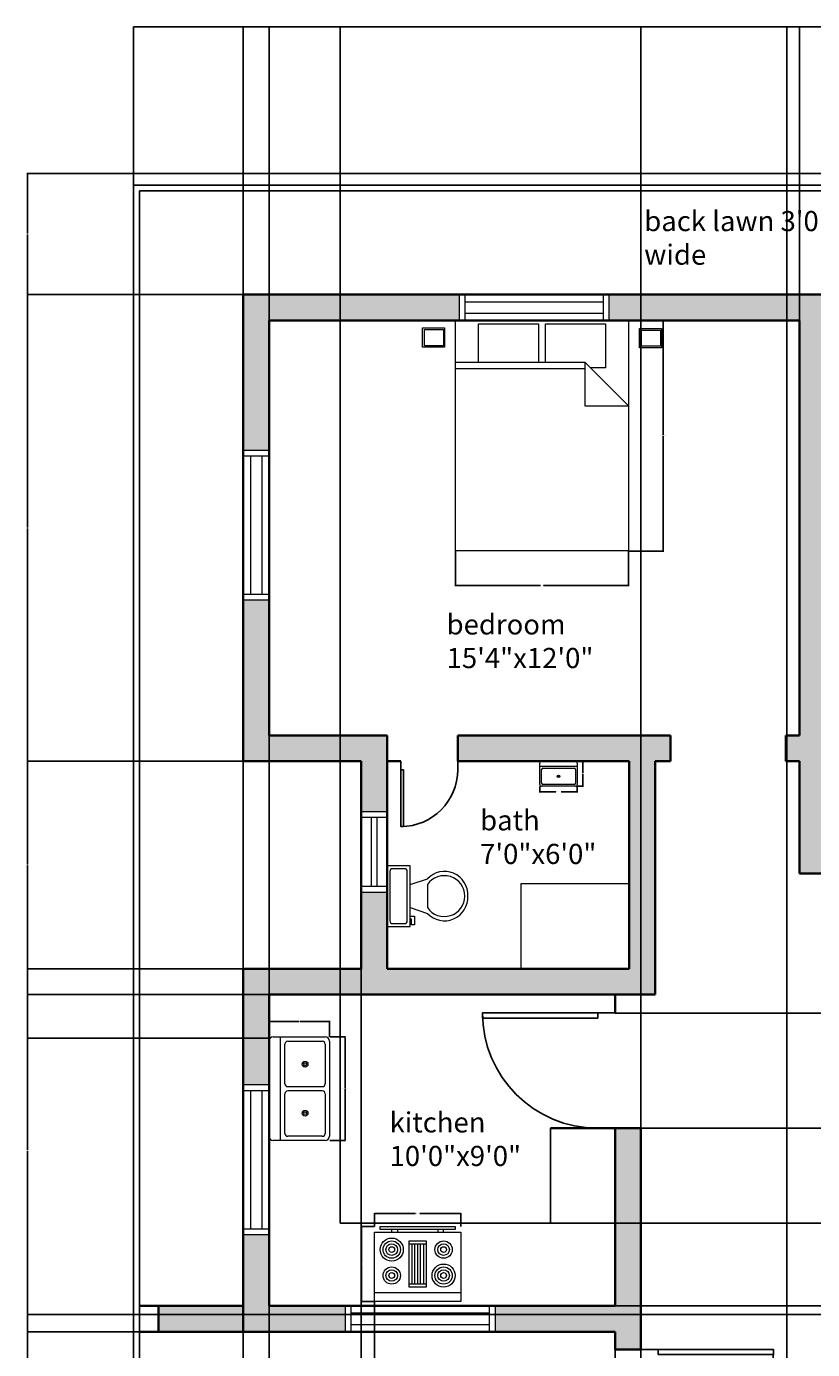
# Model space of a CAD drawing. Units: inches. Extents: x 1801 to 2333, y 478 to 1258.
# Tile 2 of 3: x 1801 to 2074, y 798 to 1258. Entities that reach past the tile are written whole.
import ezdxf

# ---------------------------------------------------------------- set-up
doc = ezdxf.new("R2010")
doc.units = ezdxf.units.IN
doc.header["$MEASUREMENT"] = 0
for name, color, linetype, lineweight in [('A-ANNO-DIMS', 2, 'Continuous', 18), ('A-AREA-IDEN', 7, 'Continuous', 18), ('A-DOOR', 4, 'Continuous', 25), ('A-EQPM', 8, 'Continuous', 18), ('A-FLOR-CASE', 8, 'Continuous', 25), ('A-FLOR-FIXT', 9, 'Continuous', 18), ('A-FURN', 8, 'Continuous', 18), ('A-GLAZ', 4, 'Continuous', 18), ('A-WALL', 7, 'Continuous', 35), ('A-WALL-PATT', 252, 'Continuous', 13), ('C-PROP', 3, 'Continuous', 25)]:
    doc.layers.add(name, color=color, linetype=linetype, lineweight=lineweight)
doc.styles.get("Standard").update_dxf_attribs({"font": 'arial.ttf'})
doc.dimstyles.get("Standard").update_dxf_attribs({"dimtxt": 0.18, "dimasz": 0.18, "dimexe": 0.18, "dimexo": 0.0625, "dimgap": 0.09, "dimtad": 0, "dimtih": 1, "dimtoh": 1, "dimdec": 0, "dimzin": 0, "dimdsep": 46, "dimlunit": 3, "dimtxsty": 'Standard', "dimcen": 0.09, "dimadec": 0, "dimazin": 0, "dimtfac": 1, "dimtdec": 0, "dimtofl": 0, "dimtmove": 0, "dimatfit": 3, "dimfxl": 1, "dimtolj": 1, "dimtzin": 0, "dimarcsym": 0})

# ---------------------------------------------------------------- blocks, each defined once
blk = doc.blocks.new('*U2')
for p, q in [((0, 0), (0, -6)), ((40, 0), (40, -6))]:
    blk.add_line(p, q)
blk.add_lwpolyline([(0, 0), (0, 40), (1.75, 40), (1.75, 0)], close=True)
blk.add_arc((0, 0), 40, 0, 90)
blk = doc.blocks.new('*U6')
for p, q in [((241.3, -152.4), (241.3, -50.8)), ((-254, -215.9), (-203.2, -215.9)), ((-254, -241.3), (-254, -215.9)), ((-203.2, -215.9), (-203.2, -203.2)), ((-177.8, -203.2), (-177.8, -241.3)), ((-101.6, -203.2), (-152.4, -355.6)), ((101.6, -203.2), (152.4, -355.6)), ((-177.8, -241.3), (-254, -241.3)), ((101.6, -355.6), (-101.6, -355.6))]:
    blk.add_line(p, q)
blk.add_lwpolyline([(266.7, -203.2), (266.7, 0), (-266.7, 0), (-266.7, -203.2)], close=True)
for points in [[(-241.3, -50.8), (-241.3, -152.4)], [(215.9, -25.4), (-215.9, -25.4)], [(-215.9, -177.8), (215.9, -177.8)]]:
    blk.add_lwpolyline(points)
for centre, radius, start, end in [((-219.075, -47.625), 22.45064, 81.8699, 188.1301), ((219.075, -47.625), 22.45064, 351.8699, 98.1301), ((-219.075, -155.575), 22.45064, 171.869898, 278.1301), ((219.075, -155.575), 22.45064, 261.8699, 8.1301), ((-12.12088, -505.93752), 205.61935, 133.01722, 273.38), ((0.94996, -504.77674), 181.02486, 124.50543, 269.7), ((-0.94742, -504.77674), 181.02486, 270.3, 55.4946), ((12.12342, -505.93752), 205.61935, 266.62, 46.9828)]:
    blk.add_arc(centre, radius, start, end)
blk = doc.blocks.new('Bed - Queen')
for p, q in [((0, -80.00003), (0, 0)), ((0, 0), (59.99999, 0)), ((59.99999, 0), (59.99999, -80.00003)), ((7.99999, -1.2), (28.79998, -1.2)), ((7.99999, -14.4), (7.99999, -1.2)), ((28.79998, -1.2), (28.79998, -14.4)), ((31.19999, -1.2), (51.99999, -1.2)), ((31.19999, -14.4), (31.19999, -1.2)), ((51.99999, -1.2), (51.99999, -16.4)), ((0, -14.4), (44.8, -14.4)), ((44.8, -16.8), (0, -16.8)), ((59.99999, -29.6), (44.8, -14.4)), ((44.8, -14.4), (44.8, -29.6)), ((51.99999, -16.4), (46.79936, -16.4)), ((44.8, -29.6), (59.99999, -29.6)), ((59.99999, -80.00003), (0, -80.00003))]:
    blk.add_line(p, q)
blk = doc.blocks.new('Sink-double - 36 in top')
for p, q in [((-18, -4), (18, -4)), ((-0.75, -18.5), (-0.75, -6.5)), ((0.75, -6.5), (0.75, -18.5))]:
    blk.add_line(p, q)
for points in [[(-16.5, 0), (16.5, 0)], [(-18, -19.5), (-18, -1.5)], [(18, -1.5), (18, -19.5)], [(-16.5, -18.5), (-16.5, -6.5)], [(-15.5, -5.5), (-1.75, -5.5)], [(1.75, -5.5), (15.5, -5.5)], [(16.5, -6.5), (16.5, -18.5)], [(16.5, -21), (-16.5, -21)], [(-1.75, -19.5), (-15.5, -19.5)], [(15.5, -19.5), (1.75, -19.5)]]:
    blk.add_lwpolyline(points)
for centre, radius in [((-8.5, -12.5), 1), ((-8.5, -12.5), 0.5), ((8.5, -12.5), 1), ((8.5, -12.5), 0.5)]:
    blk.add_circle(centre, radius)
for centre, radius, start, end in [((-16.5, -1.5), 1.5, 90, 180), ((16.5, -1.5), 1.5, 0, 90), ((-15.5, -6.5), 1, 90, 180), ((-1.75, -6.5), 1, 0, 90), ((1.75, -6.5), 1, 90, 180), ((15.5, -6.5), 1, 0, 90), ((-16.5, -19.5), 1.5, 180, 270), ((-15.5, -18.5), 1, 180, 270), ((-1.75, -18.5), 1, 270, 0), ((1.75, -18.5), 1, 180, 270), ((15.5, -18.5), 1, 270, 0), ((16.5, -19.5), 1.5, 270, 0)]:
    blk.add_arc(centre, radius, start, end)
blk = doc.blocks.new('Range-Oven - 30 in top')
for p, q in [((0, -3), (30, -3)), ((12, -6), (18, -6)), ((13, -20), (13, -6)), ((14, -6), (14, -20)), ((15, -20), (15, -6)), ((16, -6), (16, -20)), ((17, -20), (17, -6)), ((18, -20), (12, -20)), ((6, -24), (6, -25)), ((8, -25), (8, -24)), ((22, -25), (22, -24)), ((24, -24), (24, -25))]:
    blk.add_line(p, q)
for points in [[(0, -24), (0, 0), (30, 0), (30, -24)], [(12, -21), (12, -5), (18, -5), (18, -21)], [(2, -26), (2, -25), (28, -25), (28, -26)]]:
    blk.add_lwpolyline(points, close=True)
for centre, radius in [((6, -9), 4), ((6, -9), 3), ((6, -9), 2), ((6, -9), 1), ((24, -9), 3), ((24, -9), 2), ((24, -9), 1), ((6, -18), 3), ((6, -18), 2), ((6, -18), 1), ((24, -18), 4), ((24, -18), 3), ((24, -18), 2), ((24, -18), 1)]:
    blk.add_circle(centre, radius)
blk = doc.blocks.new('Sink-single - 30 in top')
blk.add_line((-15, -3.999996), (15, -3.999996))
for points in [[(-13.5, 0), (13.5, 0)], [(-15, -18.499996), (-15, -1.5)], [(-13.5, -17.499996), (-13.5, -6.499996)], [(-12.5, -5.499996), (12.5, -5.499996)], [(13.5, -6.499996), (13.5, -17.499996)], [(15, -1.5), (15, -18.499996)], [(13.5, -19.999996), (-13.5, -19.999996)], [(12.5, -18.499996), (-12.5, -18.499996)]]:
    blk.add_lwpolyline(points)
for radius in [1, 0.5]:
    blk.add_circle((0, -11.999996), radius)
for centre, radius, start, end in [((-13.5, -1.5), 1.5, 90, 180), ((-12.5, -6.499996), 1, 90, 180), ((12.5, -6.499996), 1, 0, 90), ((13.5, -1.5), 1.5, 0, 90), ((-13.5, -18.499996), 1.5, 180, 270), ((-12.5, -17.499996), 1, 180, 270), ((12.5, -17.499996), 1, 270, 0), ((13.5, -18.499996), 1.5, 270, 0)]:
    blk.add_arc(centre, radius, start, end)
blk = doc.blocks.new('WIN-48IN')
for p, q in [((0, 0), (0, 9)), ((2, 0), (2, 9)), ((2, 6.5), (50, 6.5)), ((50, 0), (50, 9)), ((52, 0), (52, 9)), ((2, 2.5), (50, 2.5))]:
    blk.add_line(p, q)
blk = doc.blocks.new('WIN-24IN')
for p, q in [((9, 28), (0, 28)), ((9, 26), (0, 26)), ((3.5, 26), (3.5, 2)), ((5.5, 26), (5.5, 2)), ((9, 2), (0, 2)), ((9, 0), (0, 0))]:
    blk.add_line(p, q)
blk = doc.blocks.new('BEDSIDE-STAND')
for points in [[(0, 6.71), (7.61, 6.71), (7.61, 0), (0, 0)], [(0.62, 6.12), (7.2, 6.12), (7.2, 0.48), (0.62, 0.48)]]:
    blk.add_lwpolyline(points, close=True)
blk = doc.blocks.new('*D23')
at = {"layer": 'A-ANNO-DIMS', "color": 0, "lineweight": -2, "transparency": 16777216}
for p, q in [((2010.04, 1155.47), (2022.16, 1155.47)), ((2021.98, 1155.29), (2021.98, 1115.66)), ((2021.98, 1075.65), (2021.98, 1115.29)), ((2010.04, 1075.47), (2022.16, 1075.47))]:
    blk.add_line(p, q, dxfattribs=at)
at = {"layer": 'A-ANNO-DIMS', "color": 0, "transparency": 16777216}
for points in [[(2021.95, 1155.29), (2022.01, 1155.29), (2021.98, 1155.47)], [(2021.95, 1075.65), (2022.01, 1075.65), (2021.98, 1075.47)]]:
    blk.add_solid(points, dxfattribs=at)
at = {"layer": 'Defpoints', "color": 0, "transparency": 16777216}
for p in [(2009.98, 1155.47), (2021.98, 1155.47), (2009.98, 1075.47)]:
    blk.add_point(p, dxfattribs=at)
at = {"layer": 'A-ANNO-DIMS', "color": 0, "transparency": 16777216, "insert": (2021.98, 1115.47), "char_height": 0.18, "attachment_point": 5}
blk.add_mtext('\\A1;QUEEN BED 80 TYP.', dxfattribs=at)
blk = doc.blocks.new('*D24')
at = {"layer": 'A-ANNO-DIMS', "color": 0, "lineweight": -2, "transparency": 16777216}
for p, q in [((1949.98, 1075.41), (1949.98, 1063.29)), ((2009.98, 1075.41), (2009.98, 1063.29)), ((1950.16, 1063.47), (1979.45, 1063.47)), ((2009.8, 1063.47), (1980.51, 1063.47))]:
    blk.add_line(p, q, dxfattribs=at)
at = {"layer": 'A-ANNO-DIMS', "color": 0, "transparency": 16777216}
for points in [[(1950.16, 1063.5), (1950.16, 1063.44), (1949.98, 1063.47)], [(2009.8, 1063.5), (2009.8, 1063.44), (2009.98, 1063.47)]]:
    blk.add_solid(points, dxfattribs=at)
at = {"layer": 'Defpoints', "color": 0, "transparency": 16777216}
for p in [(1949.98, 1075.47), (2009.98, 1075.47), (2009.98, 1063.47)]:
    blk.add_point(p, dxfattribs=at)
at = {"layer": 'A-ANNO-DIMS', "color": 0, "transparency": 16777216, "insert": (1979.98, 1063.47), "char_height": 0.18, "attachment_point": 5}
blk.add_mtext('\\A1;60 TYP.', dxfattribs=at)
blk = doc.blocks.new('*D29')
at = {"layer": 'A-ANNO-DIMS', "color": 0, "lineweight": -2, "transparency": 16777216}
for p, q in [((1979.19, 993.75), (1979.19, 991.68)), ((1992.19, 993.75), (1992.19, 991.68)), ((1979.37, 991.86), (1984.75, 991.86)), ((1992.01, 991.86), (1986.62, 991.86))]:
    blk.add_line(p, q, dxfattribs=at)
at = {"layer": 'A-ANNO-DIMS', "color": 0, "transparency": 16777216}
for points in [[(1979.37, 991.89), (1979.37, 991.83), (1979.19, 991.86)], [(1992.01, 991.89), (1992.01, 991.83), (1992.19, 991.86)]]:
    blk.add_solid(points, dxfattribs=at)
at = {"layer": 'Defpoints', "color": 0, "transparency": 16777216}
for p in [(1979.19, 993.81), (1992.19, 993.81), (1992.19, 991.86)]:
    blk.add_point(p, dxfattribs=at)
at = {"layer": 'A-ANNO-DIMS', "color": 0, "transparency": 16777216, "insert": (1985.69, 991.86), "char_height": 0.18, "attachment_point": 5}
blk.add_mtext('\\A1;BASIN 13 TYP.', dxfattribs=at)
blk = doc.blocks.new('*D30')
at = {"layer": 'A-ANNO-DIMS', "color": 0, "lineweight": -2, "transparency": 16777216}
for p, q in [((1992.25, 1002.47), (1994.32, 1002.47)), ((1994.14, 1002.29), (1994.14, 998.32)), ((1994.14, 993.99), (1994.14, 997.96)), ((1992.25, 993.81), (1994.32, 993.81))]:
    blk.add_line(p, q, dxfattribs=at)
at = {"layer": 'A-ANNO-DIMS', "color": 0, "transparency": 16777216}
for points in [[(1994.11, 1002.29), (1994.17, 1002.29), (1994.14, 1002.47)], [(1994.11, 993.99), (1994.17, 993.99), (1994.14, 993.81)]]:
    blk.add_solid(points, dxfattribs=at)
at = {"layer": 'Defpoints', "color": 0, "transparency": 16777216}
for p in [(1992.19, 1002.47), (1994.14, 1002.47), (1992.19, 993.81)]:
    blk.add_point(p, dxfattribs=at)
at = {"layer": 'A-ANNO-DIMS', "color": 0, "transparency": 16777216, "insert": (1994.14, 998.14), "char_height": 0.18, "attachment_point": 5}
blk.add_mtext('\\A1;9 TYP.', dxfattribs=at)
blk = doc.blocks.new('*D31')
at = {"layer": 'A-ANNO-DIMS', "color": 0, "lineweight": -2, "transparency": 16777216}
for p, q in [((1921.82, 841.04), (1921.82, 845.65)), ((1922, 845.47), (1936.13, 845.47)), ((1951.64, 845.47), (1937.52, 845.47)), ((1951.82, 841.04), (1951.82, 845.65))]:
    blk.add_line(p, q, dxfattribs=at)
at = {"layer": 'A-ANNO-DIMS', "color": 0, "transparency": 16777216}
for points in [[(1922, 845.5), (1922, 845.44), (1921.82, 845.47)], [(1951.64, 845.5), (1951.64, 845.44), (1951.82, 845.47)]]:
    blk.add_solid(points, dxfattribs=at)
at = {"layer": 'Defpoints', "color": 0, "transparency": 16777216}
for p in [(1921.82, 845.47), (1921.82, 840.97), (1951.82, 840.97)]:
    blk.add_point(p, dxfattribs=at)
at = {"layer": 'A-ANNO-DIMS', "color": 0, "transparency": 16777216, "insert": (1936.82, 845.47), "char_height": 0.18, "attachment_point": 5}
blk.add_mtext('\\A1;RANGE 30', dxfattribs=at)
blk = doc.blocks.new('*D32')
at = {"layer": 'A-ANNO-DIMS', "color": 0, "lineweight": -2, "transparency": 16777216}
for p, q in [((1921.76, 840.97), (1917.14, 840.97)), ((1917.32, 840.79), (1917.32, 828.16)), ((1917.32, 815.15), (1917.32, 827.79)), ((1921.76, 814.97), (1917.14, 814.97))]:
    blk.add_line(p, q, dxfattribs=at)
at = {"layer": 'A-ANNO-DIMS', "color": 0, "transparency": 16777216}
for points in [[(1917.29, 840.79), (1917.35, 840.79), (1917.32, 840.97)], [(1917.29, 815.15), (1917.35, 815.15), (1917.32, 814.97)]]:
    blk.add_solid(points, dxfattribs=at)
at = {"layer": 'Defpoints', "color": 0, "transparency": 16777216}
for p in [(1921.82, 840.97), (1917.32, 814.97), (1921.82, 814.97)]:
    blk.add_point(p, dxfattribs=at)
at = {"layer": 'A-ANNO-DIMS', "color": 0, "transparency": 16777216, "insert": (1917.32, 827.97), "char_height": 0.18, "attachment_point": 5}
blk.add_mtext('\\A1;26', dxfattribs=at)
blk = doc.blocks.new('*D33')
at = {"layer": 'A-ANNO-DIMS', "color": 0, "lineweight": -2, "transparency": 16777216}
for p, q in [((1906.31, 906.81), (1911.83, 906.81)), ((1911.65, 906.63), (1911.65, 889)), ((1911.65, 870.99), (1911.65, 888.63)), ((1906.31, 870.81), (1911.83, 870.81))]:
    blk.add_line(p, q, dxfattribs=at)
at = {"layer": 'A-ANNO-DIMS', "color": 0, "transparency": 16777216}
for points in [[(1911.62, 906.63), (1911.68, 906.63), (1911.65, 906.81)], [(1911.62, 870.99), (1911.68, 870.99), (1911.65, 870.81)]]:
    blk.add_solid(points, dxfattribs=at)
at = {"layer": 'Defpoints', "color": 0, "transparency": 16777216}
for p in [(1906.25, 906.81), (1911.65, 906.81), (1906.25, 870.81)]:
    blk.add_point(p, dxfattribs=at)
at = {"layer": 'A-ANNO-DIMS', "color": 0, "transparency": 16777216, "insert": (1911.65, 888.81), "char_height": 0.18, "attachment_point": 5}
blk.add_mtext('\\A1;DOUBLE SINK 36', dxfattribs=at)
blk = doc.blocks.new('*D34')
at = {"layer": 'A-ANNO-DIMS', "color": 0, "lineweight": -2, "transparency": 16777216}
for p, q in [((1885.25, 906.88), (1885.25, 912.39)), ((1885.43, 912.21), (1895.55, 912.21)), ((1906.07, 912.21), (1895.95, 912.21)), ((1906.25, 906.88), (1906.25, 912.39))]:
    blk.add_line(p, q, dxfattribs=at)
at = {"layer": 'A-ANNO-DIMS', "color": 0, "transparency": 16777216}
for points in [[(1885.43, 912.24), (1885.43, 912.18), (1885.25, 912.21)], [(1906.07, 912.24), (1906.07, 912.18), (1906.25, 912.21)]]:
    blk.add_solid(points, dxfattribs=at)
at = {"layer": 'Defpoints', "color": 0, "transparency": 16777216}
for p in [(1885.25, 912.21), (1885.25, 906.81), (1906.25, 906.81)]:
    blk.add_point(p, dxfattribs=at)
at = {"layer": 'A-ANNO-DIMS', "color": 0, "transparency": 16777216, "insert": (1895.75, 912.21), "char_height": 0.18, "attachment_point": 5}
blk.add_mtext('\\A1;21', dxfattribs=at)
blk = doc.blocks.new('*D35')
at = {"layer": 'A-ANNO-DIMS', "color": 0, "lineweight": -2, "transparency": 16777216}
for p, q in [((1838.29, 1202.54), (1838.29, 1257.55)), ((1838.47, 1257.37), (2067, 1257.37)), ((2296.11, 1257.37), (2067.58, 1257.37)), ((2296.29, 1206.54), (2296.29, 1257.55))]:
    blk.add_line(p, q, dxfattribs=at)
at = {"layer": 'A-ANNO-DIMS', "color": 0, "transparency": 16777216}
for points in [[(1838.47, 1257.4), (1838.47, 1257.34), (1838.29, 1257.37)], [(2296.11, 1257.4), (2296.11, 1257.34), (2296.29, 1257.37)]]:
    blk.add_solid(points, dxfattribs=at)
at = {"layer": 'Defpoints', "color": 0, "transparency": 16777216}
for p in [(2296.29, 1257.37), (2296.29, 1206.47), (1838.29, 1202.47)]:
    blk.add_point(p, dxfattribs=at)
at = {"layer": 'A-ANNO-DIMS', "color": 0, "transparency": 16777216, "insert": (2067.29, 1257.37), "char_height": 0.18, "attachment_point": 5}
blk.add_mtext('\\A1;458', dxfattribs=at)
blk = doc.blocks.new('*D37')
at = {"layer": 'A-ANNO-DIMS', "color": 0, "lineweight": -2, "transparency": 16777216}
for p, q in [((1840.29, 804.41), (1840.29, 478.11)), ((2005.29, 804.41), (2005.29, 478.11)), ((1840.47, 478.29), (1922.51, 478.29)), ((2005.11, 478.29), (1923.07, 478.29))]:
    blk.add_line(p, q, dxfattribs=at)
at = {"layer": 'A-ANNO-DIMS', "color": 0, "transparency": 16777216}
for points in [[(1840.47, 478.32), (1840.47, 478.26), (1840.29, 478.29)], [(2005.11, 478.32), (2005.11, 478.26), (2005.29, 478.29)]]:
    blk.add_solid(points, dxfattribs=at)
at = {"layer": 'Defpoints', "color": 0, "transparency": 16777216}
for p in [(1840.29, 804.47), (2005.29, 804.47), (2005.29, 478.29)]:
    blk.add_point(p, dxfattribs=at)
at = {"layer": 'A-ANNO-DIMS', "color": 0, "transparency": 16777216, "insert": (1922.79, 478.29), "char_height": 0.18, "attachment_point": 5}
blk.add_mtext('\\A1;165', dxfattribs=at)
blk = doc.blocks.new('*D39')
at = {"layer": 'A-ANNO-DIMS', "color": 0, "lineweight": -2, "transparency": 16777216}
for p, q in [((1876.29, 1164.54), (1876.29, 1257.55)), ((1876.47, 1257.37), (1972.51, 1257.37)), ((2069.11, 1257.37), (1973.07, 1257.37)), ((2069.29, 1155.54), (2069.29, 1257.55))]:
    blk.add_line(p, q, dxfattribs=at)
at = {"layer": 'A-ANNO-DIMS', "color": 0, "transparency": 16777216}
for points in [[(1876.47, 1257.4), (1876.47, 1257.34), (1876.29, 1257.37)], [(2069.11, 1257.4), (2069.11, 1257.34), (2069.29, 1257.37)]]:
    blk.add_solid(points, dxfattribs=at)
at = {"layer": 'Defpoints', "color": 0, "transparency": 16777216}
for p in [(2069.29, 1257.37), (1876.29, 1164.47), (2069.29, 1155.47)]:
    blk.add_point(p, dxfattribs=at)
at = {"layer": 'A-ANNO-DIMS', "color": 0, "transparency": 16777216, "insert": (1972.79, 1257.37), "char_height": 0.18, "attachment_point": 5}
blk.add_mtext('\\A1;193', dxfattribs=at)
blk = doc.blocks.new('*D40')
at = {"layer": 'A-ANNO-DIMS', "color": 0, "lineweight": -2, "transparency": 16777216}
for p, q in [((2069.29, 1155.54), (2069.29, 1257.55)), ((2069.47, 1257.37), (2131.51, 1257.37)), ((2194.11, 1257.37), (2132.07, 1257.37)), ((2194.29, 1164.54), (2194.29, 1257.55))]:
    blk.add_line(p, q, dxfattribs=at)
at = {"layer": 'A-ANNO-DIMS', "color": 0, "transparency": 16777216}
for points in [[(2069.47, 1257.4), (2069.47, 1257.34), (2069.29, 1257.37)], [(2194.11, 1257.4), (2194.11, 1257.34), (2194.29, 1257.37)]]:
    blk.add_solid(points, dxfattribs=at)
at = {"layer": 'Defpoints', "color": 0, "transparency": 16777216}
for p in [(2194.29, 1257.37), (2194.29, 1164.47), (2069.29, 1155.47)]:
    blk.add_point(p, dxfattribs=at)
at = {"layer": 'A-ANNO-DIMS', "color": 0, "transparency": 16777216, "insert": (2131.79, 1257.37), "char_height": 0.18, "attachment_point": 5}
blk.add_mtext('\\A1;125', dxfattribs=at)
blk = doc.blocks.new('*D42')
at = {"layer": 'A-ANNO-DIMS', "color": 0, "lineweight": -2, "transparency": 16777216}
for p, q in [((1876.23, 1002.47), (1801.26, 1002.47)), ((1801.44, 1002.29), (1801.44, 966.66)), ((1801.44, 930.65), (1801.44, 966.29)), ((1876.23, 930.47), (1801.26, 930.47))]:
    blk.add_line(p, q, dxfattribs=at)
at = {"layer": 'A-ANNO-DIMS', "color": 0, "transparency": 16777216}
for points in [[(1801.41, 1002.29), (1801.47, 1002.29), (1801.44, 1002.47)], [(1801.41, 930.65), (1801.47, 930.65), (1801.44, 930.47)]]:
    blk.add_solid(points, dxfattribs=at)
at = {"layer": 'Defpoints', "color": 0, "transparency": 16777216}
for p in [(1801.44, 1002.47), (1876.29, 1002.47), (1876.29, 930.47)]:
    blk.add_point(p, dxfattribs=at)
at = {"layer": 'A-ANNO-DIMS', "color": 0, "transparency": 16777216, "insert": (1801.44, 966.47), "char_height": 0.18, "attachment_point": 5}
blk.add_mtext('\\A1;72', dxfattribs=at)
blk = doc.blocks.new('*D43')
at = {"layer": 'A-ANNO-DIMS', "color": 0, "lineweight": -2, "transparency": 16777216}
for p, q in [((1876.23, 1164.47), (1801.26, 1164.47)), ((1801.44, 1164.29), (1801.44, 1083.66)), ((1801.44, 1002.65), (1801.44, 1083.29)), ((1876.23, 1002.47), (1801.26, 1002.47))]:
    blk.add_line(p, q, dxfattribs=at)
at = {"layer": 'A-ANNO-DIMS', "color": 0, "transparency": 16777216}
for points in [[(1801.41, 1164.29), (1801.47, 1164.29), (1801.44, 1164.47)], [(1801.41, 1002.65), (1801.47, 1002.65), (1801.44, 1002.47)]]:
    blk.add_solid(points, dxfattribs=at)
at = {"layer": 'Defpoints', "color": 0, "transparency": 16777216}
for p in [(1801.44, 1164.47), (1876.29, 1164.47), (1876.29, 1002.47)]:
    blk.add_point(p, dxfattribs=at)
at = {"layer": 'A-ANNO-DIMS', "color": 0, "transparency": 16777216, "insert": (1801.44, 1083.47), "char_height": 0.18, "attachment_point": 5}
blk.add_mtext('\\A1;162', dxfattribs=at)
blk = doc.blocks.new('*D44')
at = {"layer": 'A-ANNO-DIMS', "color": 0, "lineweight": -2, "transparency": 16777216}
for p, q in [((2194.23, 1206.47), (1801.26, 1206.47)), ((1801.44, 1206.29), (1801.44, 1185.66)), ((1801.44, 1164.65), (1801.44, 1185.29)), ((2194.23, 1164.47), (1801.26, 1164.47))]:
    blk.add_line(p, q, dxfattribs=at)
at = {"layer": 'A-ANNO-DIMS', "color": 0, "transparency": 16777216}
for points in [[(1801.41, 1206.29), (1801.47, 1206.29), (1801.44, 1206.47)], [(1801.41, 1164.65), (1801.47, 1164.65), (1801.44, 1164.47)]]:
    blk.add_solid(points, dxfattribs=at)
at = {"layer": 'Defpoints', "color": 0, "transparency": 16777216}
for p in [(1801.44, 1206.47), (2194.29, 1206.47), (2194.29, 1164.47)]:
    blk.add_point(p, dxfattribs=at)
at = {"layer": 'A-ANNO-DIMS', "color": 0, "transparency": 16777216, "insert": (1801.44, 1185.47), "char_height": 0.18, "attachment_point": 5}
blk.add_mtext('\\A1;42', dxfattribs=at)
blk = doc.blocks.new('*D45')
at = {"layer": 'A-ANNO-DIMS', "color": 0, "lineweight": -2, "transparency": 16777216}
for p, q in [((1876.29, 1002.41), (1876.29, 478.11)), ((1917.2, 1002.41), (1917.2, 478.11)), ((1876.47, 478.29), (1896.36, 478.29)), ((1917.02, 478.29), (1897.12, 478.29))]:
    blk.add_line(p, q, dxfattribs=at)
at = {"layer": 'A-ANNO-DIMS', "color": 0, "transparency": 16777216}
for points in [[(1876.47, 478.32), (1876.47, 478.26), (1876.29, 478.29)], [(1917.02, 478.32), (1917.02, 478.26), (1917.2, 478.29)]]:
    blk.add_solid(points, dxfattribs=at)
at = {"layer": 'Defpoints', "color": 0, "transparency": 16777216}
for p in [(1876.29, 1002.47), (1917.2, 1002.47), (1917.2, 478.29)]:
    blk.add_point(p, dxfattribs=at)
at = {"layer": 'A-ANNO-DIMS', "color": 0, "transparency": 16777216, "insert": (1896.74, 478.29), "char_height": 0.18, "attachment_point": 5}
blk.add_mtext('\\A1;40.91', dxfattribs=at)
blk = doc.blocks.new('*D48')
at = {"layer": 'A-ANNO-DIMS', "color": 0, "lineweight": -2, "transparency": 16777216}
for p, q in [((2147.23, 810.47), (1801.26, 810.47)), ((1801.44, 810.29), (1801.44, 789.42)), ((1801.44, 768.17), (1801.44, 789.05)), ((2147.23, 767.99), (1801.26, 767.99))]:
    blk.add_line(p, q, dxfattribs=at)
at = {"layer": 'A-ANNO-DIMS', "color": 0, "transparency": 16777216}
for points in [[(1801.41, 810.29), (1801.47, 810.29), (1801.44, 810.47)], [(1801.41, 768.17), (1801.47, 768.17), (1801.44, 767.99)]]:
    blk.add_solid(points, dxfattribs=at)
at = {"layer": 'Defpoints', "color": 0, "transparency": 16777216}
for p in [(1801.44, 810.47), (2147.29, 810.47), (2147.29, 767.99)]:
    blk.add_point(p, dxfattribs=at)
at = {"layer": 'A-ANNO-DIMS', "color": 0, "transparency": 16777216, "insert": (1801.44, 789.23), "char_height": 0.18, "attachment_point": 5}
blk.add_mtext('\\A1;42.48', dxfattribs=at)
blk = doc.blocks.new('*D49')
at = {"layer": 'A-ANNO-DIMS', "color": 0, "lineweight": -2, "transparency": 16777216}
for p, q in [((1876.23, 930.47), (1801.26, 930.47)), ((1801.44, 930.29), (1801.44, 867.66)), ((1801.44, 804.65), (1801.44, 867.29)), ((1876.23, 804.47), (1801.26, 804.47))]:
    blk.add_line(p, q, dxfattribs=at)
at = {"layer": 'A-ANNO-DIMS', "color": 0, "transparency": 16777216}
for points in [[(1801.41, 930.29), (1801.47, 930.29), (1801.44, 930.47)], [(1801.41, 804.65), (1801.47, 804.65), (1801.44, 804.47)]]:
    blk.add_solid(points, dxfattribs=at)
at = {"layer": 'Defpoints', "color": 0, "transparency": 16777216}
for p in [(1801.44, 930.47), (1876.29, 930.47), (1876.29, 804.47)]:
    blk.add_point(p, dxfattribs=at)
at = {"layer": 'A-ANNO-DIMS', "color": 0, "transparency": 16777216, "insert": (1801.44, 867.47), "char_height": 0.18, "attachment_point": 5}
blk.add_mtext('\\A1;126', dxfattribs=at)
blk = doc.blocks.new('*D50')
at = {"layer": 'A-ANNO-DIMS', "color": 0, "lineweight": -2, "transparency": 16777216}
for p, q in [((1885.29, 921.54), (1885.29, 1257.55)), ((1885.47, 1257.37), (1897.18, 1257.37)), ((1909.81, 1257.37), (1898.1, 1257.37)), ((1909.99, 921.54), (1909.99, 1257.55))]:
    blk.add_line(p, q, dxfattribs=at)
at = {"layer": 'A-ANNO-DIMS', "color": 0, "transparency": 16777216}
for points in [[(1885.47, 1257.4), (1885.47, 1257.34), (1885.29, 1257.37)], [(1909.81, 1257.4), (1909.81, 1257.34), (1909.99, 1257.37)]]:
    blk.add_solid(points, dxfattribs=at)
at = {"layer": 'Defpoints', "color": 0, "transparency": 16777216}
for p in [(1909.99, 1257.37), (1885.29, 921.47), (1909.99, 921.47)]:
    blk.add_point(p, dxfattribs=at)
at = {"layer": 'A-ANNO-DIMS', "color": 0, "transparency": 16777216, "insert": (1897.64, 1257.37), "char_height": 0.18, "attachment_point": 5}
blk.add_mtext('\\A1;24.704', dxfattribs=at)
blk = doc.blocks.new('*D51')
at = {"layer": 'A-ANNO-DIMS', "color": 0, "lineweight": -2, "transparency": 16777216}
for p, q in [((1982.97, 842.2), (2333.32, 842.2)), ((2333.14, 842.02), (2333.14, 828.02)), ((2333.14, 813.65), (2333.14, 827.65)), ((2005.35, 813.47), (2333.32, 813.47))]:
    blk.add_line(p, q, dxfattribs=at)
at = {"layer": 'A-ANNO-DIMS', "color": 0, "transparency": 16777216}
for points in [[(2333.11, 842.02), (2333.17, 842.02), (2333.14, 842.2)], [(2333.11, 813.65), (2333.17, 813.65), (2333.14, 813.47)]]:
    blk.add_solid(points, dxfattribs=at)
at = {"layer": 'Defpoints', "color": 0, "transparency": 16777216}
for p in [(1982.91, 842.2), (2005.29, 813.47), (2333.14, 813.47)]:
    blk.add_point(p, dxfattribs=at)
at = {"layer": 'A-ANNO-DIMS', "color": 0, "transparency": 16777216, "insert": (2333.14, 827.84), "char_height": 0.18, "attachment_point": 5}
blk.add_mtext('\\A1;28.72', dxfattribs=at)
blk = doc.blocks.new('*D52')
at = {"layer": 'A-ANNO-DIMS', "color": 0, "lineweight": -2, "transparency": 16777216}
for p, q in [((1885.29, 813.41), (1885.29, 478.11)), ((1921.82, 814.91), (1921.82, 478.11)), ((1885.47, 478.29), (1903.09, 478.29)), ((1921.64, 478.29), (1904.02, 478.29))]:
    blk.add_line(p, q, dxfattribs=at)
at = {"layer": 'A-ANNO-DIMS', "color": 0, "transparency": 16777216}
for points in [[(1885.47, 478.32), (1885.47, 478.26), (1885.29, 478.29)], [(1921.64, 478.32), (1921.64, 478.26), (1921.82, 478.29)]]:
    blk.add_solid(points, dxfattribs=at)
at = {"layer": 'Defpoints', "color": 0, "transparency": 16777216}
for p in [(1885.29, 813.47), (1921.82, 814.97), (1921.82, 478.29)]:
    blk.add_point(p, dxfattribs=at)
at = {"layer": 'A-ANNO-DIMS', "color": 0, "transparency": 16777216, "insert": (1903.56, 478.29), "char_height": 0.18, "attachment_point": 5}
blk.add_mtext('\\A1;36.534', dxfattribs=at)
blk = doc.blocks.new('*D53')
at = {"layer": 'A-ANNO-DIMS', "color": 0, "lineweight": -2, "transparency": 16777216}
for p, q in [((1885.23, 921.47), (1801.26, 921.47)), ((1801.44, 921.29), (1801.44, 914.11)), ((1801.44, 906.55), (1801.44, 913.74)), ((1885.63, 906.37), (1801.26, 906.37))]:
    blk.add_line(p, q, dxfattribs=at)
at = {"layer": 'A-ANNO-DIMS', "color": 0, "transparency": 16777216}
for points in [[(1801.41, 921.29), (1801.47, 921.29), (1801.44, 921.47)], [(1801.41, 906.55), (1801.47, 906.55), (1801.44, 906.37)]]:
    blk.add_solid(points, dxfattribs=at)
at = {"layer": 'Defpoints', "color": 0, "transparency": 16777216}
for p in [(1885.29, 921.47), (1801.44, 906.37), (1885.69, 906.37)]:
    blk.add_point(p, dxfattribs=at)
at = {"layer": 'A-ANNO-DIMS', "color": 0, "transparency": 16777216, "insert": (1801.44, 913.92), "char_height": 0.18, "attachment_point": 5}
blk.add_mtext('\\A1;15.1', dxfattribs=at)
blk = doc.blocks.new('*D54')
at = {"layer": 'A-ANNO-DIMS', "color": 0, "lineweight": -2, "transparency": 16777216}
for p, q in [((2005.35, 915.1), (2333.32, 915.1)), ((2333.14, 914.92), (2333.14, 895.29)), ((2333.14, 875.28), (2333.14, 894.92)), ((2005.35, 875.1), (2333.32, 875.1))]:
    blk.add_line(p, q, dxfattribs=at)
at = {"layer": 'A-ANNO-DIMS', "color": 0, "transparency": 16777216}
for points in [[(2333.11, 914.92), (2333.17, 914.92), (2333.14, 915.1)], [(2333.11, 875.28), (2333.17, 875.28), (2333.14, 875.1)]]:
    blk.add_solid(points, dxfattribs=at)
at = {"layer": 'Defpoints', "color": 0, "transparency": 16777216}
for p in [(2005.29, 915.1), (2333.14, 915.1), (2005.29, 875.1)]:
    blk.add_point(p, dxfattribs=at)
at = {"layer": 'A-ANNO-DIMS', "color": 0, "transparency": 16777216, "insert": (2333.14, 895.1), "char_height": 0.18, "attachment_point": 5}
blk.add_mtext('\\A1;40', dxfattribs=at)
blk = doc.blocks.new('*D55')
at = {"layer": 'A-ANNO-DIMS', "color": 0, "lineweight": -2, "transparency": 16777216}
for p, q in [((2014.29, 702.54), (2014.29, 1257.55)), ((2014.47, 1257.37), (2039.21, 1257.37)), ((2064.75, 1257.37), (2040, 1257.37)), ((2064.93, 702.54), (2064.93, 1257.55))]:
    blk.add_line(p, q, dxfattribs=at)
at = {"layer": 'A-ANNO-DIMS', "color": 0, "transparency": 16777216}
for points in [[(2014.47, 1257.4), (2014.47, 1257.34), (2014.29, 1257.37)], [(2064.75, 1257.4), (2064.75, 1257.34), (2064.93, 1257.37)]]:
    blk.add_solid(points, dxfattribs=at)
at = {"layer": 'Defpoints', "color": 0, "transparency": 16777216}
for p in [(2064.93, 1257.37), (2014.29, 702.47), (2064.93, 702.47)]:
    blk.add_point(p, dxfattribs=at)
at = {"layer": 'A-ANNO-DIMS', "color": 0, "transparency": 16777216, "insert": (2039.61, 1257.37), "char_height": 0.18, "attachment_point": 5}
blk.add_mtext('\\A1;50.64', dxfattribs=at)

msp = doc.modelspace()

# ---------------------------------------------------------------- hatches: boundary and pattern name
at = {"layer": 'A-WALL-PATT'}
h = msp.add_hatch(color=256, dxfattribs=at)
h.dxf.hatch_style = 1
h.paths.add_polyline_path([(1951.2881, 1164.4747), (1876.2881, 1164.4747), (1876.2881, 1110.5123), (1885.2881, 1110.5123), (1885.2881, 1155.4747), (1951.2881, 1155.4747)])
h.paths.add_polyline_path([(2126.8707, 1164.4747), (2003.2881, 1164.4747), (2003.2881, 1155.4747), (2069.2881, 1155.4747), (2069.2881, 1011.4747), (2064.4791, 1011.4747), (2064.4791, 1002.4747), (2069.2881, 1002.4747), (2069.2881, 963.4747), (2078.3234, 963.4747), (2086.6392, 963.4747), (2086.6392, 972.4747), (2078.3234, 972.4747), (2078.2881, 1002.4747), (2078.2881, 1155.4747), (2126.8707, 1155.4747)])
h.paths.add_polyline_path([(2194.2881, 1164.4747), (2178.8707, 1164.4747), (2178.8707, 1155.4747), (2194.2881, 1155.4747)])
h.paths.add_polyline_path([(2203.2881, 1206.4747), (2194.2881, 1206.4747), (2194.2881, 1156.4812), (2203.2881, 1156.4812)])
h.paths.add_polyline_path([(2296.2881, 1206.4747), (2287.2881, 1206.4747), (2287.2881, 1187.4062), (2296.2881, 1187.4062)])
h = msp.add_hatch(color=256, dxfattribs=at)
h.dxf.hatch_style = 1
h.paths.add_polyline_path([(1926.1982, 1011.4747), (1885.2881, 1011.4747), (1885.2881, 1058.5123), (1876.2881, 1058.5123), (1876.2881, 1002.4747), (1917.1982, 1002.4747), (1917.1982, 984.9747), (1926.1982, 984.9747)])
h.paths.add_polyline_path([(2024.4791, 1011.4747), (1950.7011, 1011.4747), (1950.7011, 1002.4747), (2010.1982, 1002.4747), (2010.1982, 930.4747), (1972.6781, 930.4747), (1926.1982, 930.4747), (1926.1982, 956.9747), (1917.1982, 956.9747), (1917.1982, 930.4747), (1876.2881, 930.4747), (1876.2881, 890.2272), (1885.2881, 890.2272), (1885.2881, 921.4747), (2014.2881, 921.4747), (2019.1982, 921.4747), (2019.1982, 1002.4747), (2024.4791, 1002.4747)])
h.paths.add_polyline_path([(1911.7913, 813.4747), (1885.2881, 813.4747), (1885.2881, 838.2272), (1876.2881, 838.2272), (1876.2881, 804.4747), (1911.7913, 804.4747)])
h.paths.add_polyline_path([(1876.2881, 813.4747), (1846.9543, 813.4747), (1846.9543, 804.4747), (1876.2881, 804.4747)])
h.paths.add_polyline_path([(2014.2881, 875.105), (2005.2881, 875.105), (2005.2881, 813.4747), (1963.7913, 813.4747), (1963.7913, 804.4747), (2005.2881, 804.4747), (2005.2881, 798.2841), (2014.2881, 798.2841), (2014.2881, 804.4747)])

# ---------------------------------------------------------------- linework, layer by layer
at = {"layer": 'A-FLOR-CASE'}
for p, q in [((1909.9916, 921.4747), (1909.9916, 842.1967)), ((1982.9092, 842.1967), (1982.9092, 875.105)), ((1909.9916, 842.1967), (1982.9092, 842.1967))]:
    msp.add_line(p, q, dxfattribs=at)
at = {"layer": 'A-FLOR-FIXT'}
msp.add_lwpolyline([(2010.1982, 930.4747), (1972.6781, 930.4747), (1972.6781, 960.0868), (2010.1982, 960.0868)], close=True, dxfattribs=at)
at = {"layer": 'A-WALL'}
for p, q in [((1876.2881, 1164.4747), (2194.2881, 1164.4747)), ((1876.2881, 1002.4747), (1876.2881, 1164.4747)), ((1885.2881, 1155.4747), (2069.2881, 1155.4747)), ((1885.2881, 1011.4747), (1885.2881, 1155.4747)), ((2069.2881, 1011.4747), (2069.2881, 1155.4747)), ((1885.2881, 1011.4747), (1926.1982, 1011.4747)), ((1926.1982, 1011.4747), (1926.1982, 930.4747)), ((1950.7011, 1011.4747), (2024.4791, 1011.4747)), ((1950.7011, 1002.4747), (1950.7011, 1011.4747)), ((2024.4791, 1011.4747), (2024.4791, 1002.4747)), ((2064.4791, 1011.4747), (2064.4791, 1002.4747)), ((2064.4791, 1011.4747), (2069.2881, 1011.4747)), ((1876.2881, 1002.4747), (1917.1982, 1002.4747)), ((1917.1982, 1002.4747), (1917.1982, 930.4747)), ((1926.1982, 1002.4747), (1931.0142, 1002.4747)), ((1950.7011, 1002.4747), (2010.1982, 1002.4747)), ((2010.1982, 1002.4747), (2010.1982, 930.4747)), ((2019.1982, 1002.4747), (2019.1982, 921.4747)), ((2019.1982, 1002.4747), (2024.4791, 1002.4747)), ((2064.4791, 1002.4747), (2069.2881, 1002.4747)), ((2069.2881, 1002.4747), (2069.2881, 963.4747)), ((2069.2881, 963.4747), (2078.3234, 963.4747)), ((1876.2881, 930.4747), (1917.1982, 930.4747)), ((1876.2881, 804.4747), (1876.2881, 930.4747)), ((1926.1982, 930.4747), (2010.1982, 930.4747)), ((1885.2881, 921.4747), (2014.2881, 921.4747)), ((1885.2881, 813.4747), (1885.2881, 921.4747)), ((2005.2881, 915.105), (2005.2881, 921.4747)), ((2014.2881, 921.4747), (2019.1982, 921.4747)), ((1982.9092, 875.105), (2014.2881, 875.105)), ((2005.2881, 813.4747), (2005.2881, 875.105)), ((2014.2881, 804.4747), (2014.2881, 875.105)), ((1840.2881, 813.4747), (1876.2881, 813.4747)), ((1846.9543, 813.4747), (1846.9543, 804.4747)), ((1885.2881, 813.4747), (2005.2881, 813.4747)), ((1840.2881, 804.4747), (1876.2881, 804.4747)), ((1876.2881, 804.4747), (2005.2881, 804.4747)), ((2005.2881, 804.4747), (2005.2881, 798.2841)), ((2014.2881, 804.4747), (2014.2881, 798.2841)), ((2014.2881, 798.2841), (2005.2881, 798.2841))]:
    msp.add_line(p, q, dxfattribs=at)
at = {"layer": 'C-PROP'}
for p, q in [((1838.2881, 1002.4747), (1838.2881, 1202.4747)), ((1838.2881, 1202.4747), (2194.2881, 1202.4747)), ((1840.2881, 1002.4747), (1840.2881, 1200.4747)), ((1840.2881, 1200.4747), (2194.2881, 1200.4747)), ((1838.2881, 1002.4747), (1838.2881, 930.4747)), ((1840.2881, 1002.4747), (1840.2881, 930.4747)), ((1838.2881, 515.4747), (1838.2881, 930.4747)), ((1840.2881, 517.4747), (1840.2881, 930.4747))]:
    msp.add_line(p, q, dxfattribs=at)

# ---------------------------------------------------------------- block references
at = {"layer": 'A-DOOR', "xscale": -0.4921731194801604, "yscale": 0.4921731194801604, "zscale": 0.4921731194801604, "rotation": 180}
msp.add_blockref('*U2', (1931.0142, 999.5217), dxfattribs=at)
at = {"layer": 'A-DOOR', "xscale": -1, "rotation": 90}
msp.add_blockref('*U2', (1999.2881, 915.105), dxfattribs=at)
at = {"layer": 'A-DOOR', "rotation": 270}
msp.add_blockref('*U2', (2020.2881, 798.2841), dxfattribs=at)
at = {"layer": 'A-EQPM', "rotation": 180}
msp.add_blockref('Range-Oven - 30 in top', (1951.8221, 814.9737), dxfattribs=at)
at = {"layer": 'A-FLOR-FIXT', "xscale": 0.4333333333333334, "yscale": 0.4333333333333334, "zscale": 0.4333333333333334}
msp.add_blockref('Sink-single - 30 in top', (1985.6856, 1002.4747), dxfattribs=at)
at = {"layer": 'A-FLOR-FIXT', "xscale": 0.0393700787401575, "yscale": 0.0393700787401575, "zscale": 0.0393700787401575, "rotation": 90}
msp.add_blockref('*U6', (1926.1982, 955.684), dxfattribs=at)
at = {"layer": 'A-FLOR-FIXT', "rotation": 90}
msp.add_blockref('Sink-double - 36 in top', (1885.2517, 888.8131), dxfattribs=at)
at = {"layer": 'A-FURN'}
for name, p in [('BEDSIDE-STAND', (1938.5554, 1146.225)), ('Bed - Queen', (1949.977, 1155.4747)), ('BEDSIDE-STAND', (2013.818, 1146.043))]:
    msp.add_blockref(name, p, dxfattribs=at)
at = {"layer": 'A-GLAZ'}
for name, p in [('WIN-48IN', (1951.288, 1155.475)), ('WIN-24IN', (1917.198, 956.975)), ('WIN-48IN', (1911.7912, 804.475))]:
    msp.add_blockref(name, p, dxfattribs=at)
for p, rotation in [((1876.2883, 1110.5123), 270.0000000000017), ((1876.2883, 890.2273), 270.0000000000006)]:
    msp.add_blockref('WIN-48IN', p, dxfattribs=dict(at, rotation=rotation))

# ---------------------------------------------------------------- texts
at = {"layer": 'A-AREA-IDEN', "char_height": 7, "attachment_point": 1}
for s, width, insert in [('back lawn 3\'0" wide', 84.800625, (2015.4244, 1193.499)), ('bedroom\\P15\'4"x12\'0"\\P  ', 106.765691, (1946.8666, 1053.4901)), ('bath\\P7\'0"x6\'0"\\P  ', 106.765691, (1958.4955, 985.4896)), ('kitchen\\P10\'0"x9\'0"\\P  ', 106.765691, (1927.0766, 880.6473))]:
    msp.add_mtext_dynamic_manual_height_columns(s, width=width, gutter_width=1, heights=[0], dxfattribs=dict(at, insert=insert))

# ---------------------------------------------------------------- dimensions: what is measured, and where the dimension line sits
at = {"layer": 'A-ANNO-DIMS'}
for base, p1, p2, override, picture, middle in [((2296.2881, 1257.3702), (1838.2881, 1202.4747), (2296.2881, 1206.4747), {"dimdec": 0, "dimlfac": 1, "dimrnd": 0, "dimzin": 0, "dimdsep": 46, "dimlunit": 2}, '*D35', (2067.2881, 1257.3702)), ((2069.2881, 1257.3702), (1876.2881, 1164.4747), (2069.2881, 1155.4747), {"dimdec": 0, "dimlfac": 1, "dimrnd": 0, "dimzin": 0, "dimdsep": 46, "dimlunit": 2}, '*D39', (1972.7881, 1257.3702)), ((1909.99162, 1257.37018), (1885.28807, 921.47475), (1909.99162, 921.47475), {"dimdec": 3, "dimlfac": 1, "dimrnd": 0, "dimzin": 0, "dimdsep": 46, "dimlunit": 2}, '*D50', (1897.63985, 1257.37018)), ((2064.9263, 1257.3702), (2014.2881, 702.4747), (2064.9263, 702.4747), {"dimdec": 2, "dimlfac": 1, "dimrnd": 0, "dimzin": 0, "dimdsep": 46, "dimlunit": 2}, '*D55', (2039.6072, 1257.3702)), ((2194.2881, 1257.3702), (2069.2881, 1155.4747), (2194.2881, 1164.4747), {"dimdec": 0, "dimlfac": 1, "dimrnd": 0, "dimzin": 0, "dimdsep": 46, "dimlunit": 2}, '*D40', (2131.7881, 1257.3702)), ((1917.1982, 478.2946), (1876.2881, 1002.4747), (1917.1982, 1002.4747), {"dimdec": 2, "dimlfac": 1, "dimrnd": 0, "dimzin": 0, "dimdsep": 46, "dimlunit": 2}, '*D45', (1896.7431, 478.2946)), ((1921.8221, 478.2946), (1885.2881, 813.4747), (1921.8221, 814.9737), {"dimdec": 3, "dimlfac": 1, "dimrnd": 0, "dimzin": 0, "dimdsep": 46, "dimlunit": 2}, '*D52', (1903.5551, 478.2946)), ((2005.2881, 478.2946), (1840.2881, 804.4747), (2005.2881, 804.4747), {"dimdec": 0, "dimlfac": 1, "dimrnd": 0, "dimzin": 0, "dimdsep": 46, "dimlunit": 2}, '*D37', (1922.7881, 478.2946))]:
    dim = msp.add_linear_dim(base=base, p1=p1, p2=p2, dimstyle='Standard', override=override, dxfattribs=at)
    dim.commit()
    dim.dimension.update_dxf_attribs({"geometry": picture, "text_midpoint": middle})
for base, p1, p2, angle, override, picture, middle in [((1801.4381, 1206.4747), (2194.2881, 1164.4747), (2194.2881, 1206.4747), 90, {"dimdec": 0, "dimlfac": 1, "dimrnd": 0, "dimzin": 0, "dimdsep": 46, "dimlunit": 2}, '*D44', (1801.4381, 1185.4747)), ((1801.4381, 1164.4747), (1876.2881, 1002.4747), (1876.2881, 1164.4747), 90, {"dimdec": 0, "dimlfac": 1, "dimrnd": 0, "dimzin": 0, "dimdsep": 46, "dimlunit": 2}, '*D43', (1801.4381, 1083.4747)), ((1801.4381, 1002.4747), (1876.2881, 930.4747), (1876.2881, 1002.4747), 90, {"dimdec": 0, "dimlfac": 1, "dimrnd": 0, "dimzin": 0, "dimdsep": 46, "dimlunit": 2}, '*D42', (1801.4381, 966.4747)), ((1801.4381, 930.4747), (1876.2881, 804.4747), (1876.2881, 930.4747), 90, {"dimdec": 0, "dimlfac": 1, "dimrnd": 0, "dimzin": 0, "dimdsep": 46, "dimlunit": 2}, '*D49', (1801.4381, 867.4747)), ((1801.4381, 906.3738), (1885.2881, 921.4747), (1885.691, 906.3738), 90, {"dimdec": 1, "dimlfac": 1, "dimrnd": 0, "dimzin": 0, "dimdsep": 46, "dimlunit": 2}, '*D53', (1801.4381, 913.9243)), ((2333.1381, 915.105), (2005.2881, 875.105), (2005.2881, 915.105), 90, {"dimdec": 0, "dimlfac": 1, "dimrnd": 0, "dimzin": 0, "dimdsep": 46, "dimlunit": 2}, '*D54', (2333.1381, 895.105)), ((1885.2517, 912.2131), (1906.2517, 906.8131), (1885.2517, 906.8131), 180, {"dimdec": 0, "dimlfac": 1, "dimrnd": 0, "dimzin": 0, "dimdsep": 46, "dimlunit": 2}, '*D34', (1895.7517, 912.2131)), ((1917.3221, 814.9737), (1921.8221, 840.9737), (1921.8221, 814.9737), 270, {"dimdec": 0, "dimlfac": 1, "dimrnd": 0, "dimzin": 0, "dimdsep": 46, "dimlunit": 2}, '*D32', (1917.3221, 827.9737)), ((2333.1381, 813.4747), (1982.9092, 842.1967), (2005.2881, 813.4747), 90, {"dimdec": 2, "dimlfac": 1, "dimrnd": 0, "dimzin": 0, "dimdsep": 46, "dimlunit": 2}, '*D51', (2333.1381, 827.8357)), ((1801.4381, 810.4747), (2147.2881, 767.9929), (2147.2881, 810.4747), 90, {"dimdec": 2, "dimlfac": 1, "dimrnd": 0, "dimzin": 0, "dimdsep": 46, "dimlunit": 2}, '*D48', (1801.4381, 789.2338))]:
    dim = msp.add_linear_dim(base=base, p1=p1, p2=p2, angle=angle, dimstyle='Standard', override=override, dxfattribs=at)
    dim.commit()
    dim.dimension.update_dxf_attribs({"geometry": picture, "text_midpoint": middle})
for base, p1, p2, angle, text, picture, middle in [((2021.977, 1155.4747), (2009.977, 1075.4747), (2009.977, 1155.4747), 90, 'QUEEN BED <> TYP.', '*D23', (2021.977, 1115.4747)), ((1994.1356, 1002.4747), (1992.1856, 993.8081), (1992.1856, 1002.4747), 90, '<> TYP.', '*D30', (1994.1356, 998.1414)), ((1911.6517, 906.8131), (1906.2517, 870.8131), (1906.2517, 906.8131), 90, 'DOUBLE SINK <>', '*D33', (1911.6517, 888.8131)), ((1921.8221, 845.4737), (1951.8221, 840.9737), (1921.8221, 840.9737), 180, 'RANGE <>', '*D31', (1936.8221, 845.4737))]:
    dim = msp.add_linear_dim(base=base, p1=p1, p2=p2, angle=angle, text=text, dimstyle='Standard', override={"dimdec": 0, "dimlfac": 1, "dimrnd": 0, "dimzin": 0, "dimdsep": 46, "dimlunit": 2}, dxfattribs=at)
    dim.commit()
    dim.dimension.update_dxf_attribs({"geometry": picture, "text_midpoint": middle})
for base, p1, p2, text, picture, middle in [((2009.977, 1063.4747), (1949.977, 1075.4747), (2009.977, 1075.4747), '<> TYP.', '*D24', (1979.977, 1063.4747)), ((1992.1856, 991.8581), (1979.1856, 993.8081), (1992.1856, 993.8081), 'BASIN <> TYP.', '*D29', (1985.6856, 991.8581))]:
    dim = msp.add_linear_dim(base=base, p1=p1, p2=p2, text=text, dimstyle='Standard', override={"dimdec": 0, "dimlfac": 1, "dimrnd": 0, "dimzin": 0, "dimdsep": 46, "dimlunit": 2}, dxfattribs=at)
    dim.commit()
    dim.dimension.update_dxf_attribs({"geometry": picture, "text_midpoint": middle})

doc.saveas('drawing.dxf')
